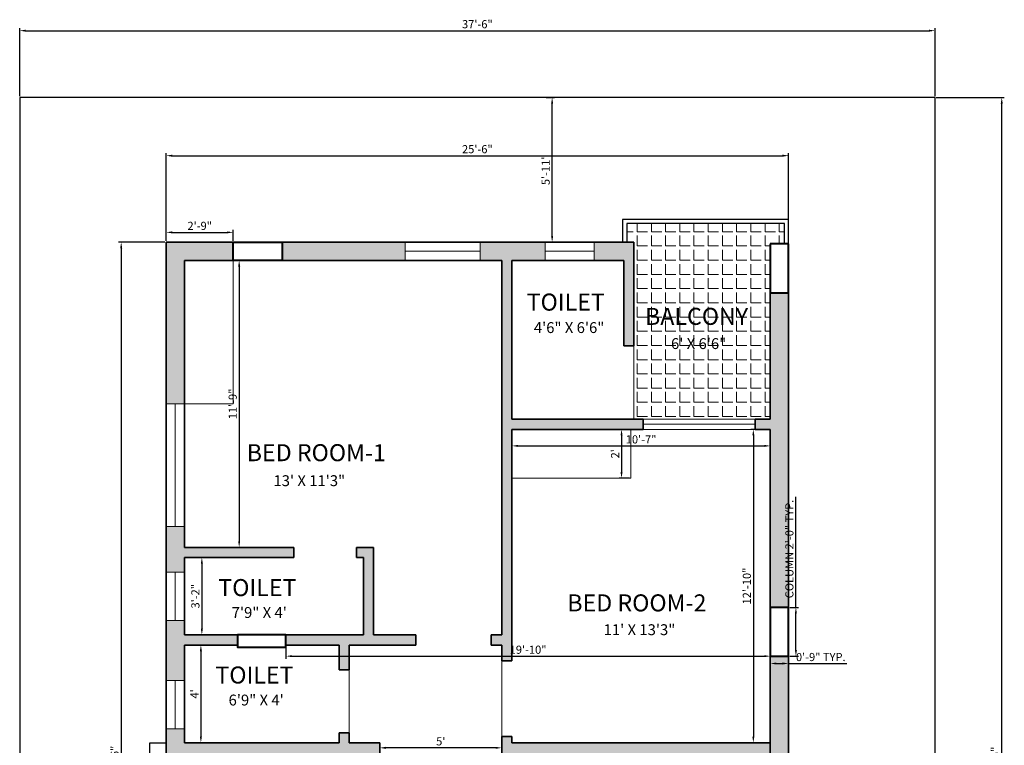
# Model space of a CAD drawing. Units: millimetres. Extents: x 2190 to 2674, y 1487 to 2179.
# Tile 2 of 2: x 2190 to 2674, y 1822 to 2179. Entities that reach past the tile are written whole.
import ezdxf

# ---------------------------------------------------------------- set-up
doc = ezdxf.new("R2010")
doc.units = ezdxf.units.MM
for name, color, linetype, lineweight in [('A-ANNO-DIMS', 2, 'Continuous', 18), ('A-AREA-IDEN', 7, 'Continuous', 18), ('A-WALL', 7, 'Continuous', 35), ('C-PROP', 7, 'Continuous', 25)]:
    doc.layers.add(name, color=color, linetype=linetype, lineweight=lineweight)
for name, color, linetype, lineweight, true_color in [('A-COLS', 240, 'Continuous', 40, 0xed1f24), ('A-DOOR', 177, 'Continuous', 18, 0x293189), ('A-FLOR-CASE', 177, 'Continuous', 18, 0x293189), ('A-FLOR-HRAL', 177, 'Continuous', 25, 0x293189), ('A-FLOR-PATT', 252, 'Continuous', 13, 0x939598), ('A-GLAZ', 177, 'Continuous', 18, 0x293189), ('A-WALL-PATT', 32, 'Continuous', 13, 0xcd6928)]:
    doc.layers.add(name, color=color, linetype=linetype, lineweight=lineweight, true_color=true_color)
doc.styles.get("Standard").update_dxf_attribs({"font": 'arial.ttf'})
doc.dimstyles.new('ISO-25', dxfattribs={"dimtxt": 4, "dimasz": 3, "dimexe": 1.25, "dimexo": 0.625, "dimtad": 1, "dimdec": 0, "dimlunit": 3, "dimtxsty": 'Standard', "dimcen": 2.5, "dimadec": 0, "dimazin": 0, "dimtfac": 1, "dimtdec": 0, "dimtmove": 0, "dimatfit": 3, "dimfxl": 1, "dimarcsym": 0})

# ---------------------------------------------------------------- blocks, each defined once
blk = doc.blocks.new('*D1')
at = {"layer": 'A-ANNO-DIMS', "color": 0, "lineweight": -2, "transparency": 16777216}
for p, q in [((2295.73, 2060.45), (2299.26, 2060.45)), ((2298.01, 2057.45), (2298.01, 1922.45)), ((2295.73, 1919.45), (2299.26, 1919.45))]:
    blk.add_line(p, q, dxfattribs=at)
at = {"layer": 'A-ANNO-DIMS', "color": 0, "transparency": 16777216}
for points in [[(2297.51, 2057.45), (2298.51, 2057.45), (2298.01, 2060.45)], [(2297.51, 1922.45), (2298.51, 1922.45), (2298.01, 1919.45)]]:
    blk.add_solid(points, dxfattribs=at)
at = {"layer": 'Defpoints', "color": 0, "transparency": 16777216}
for p in [(2295.11, 2060.45), (2295.11, 1919.45), (2298.01, 1919.45)]:
    blk.add_point(p, dxfattribs=at)
at = {"layer": 'A-ANNO-DIMS', "color": 0, "transparency": 16777216, "insert": (2295.35, 1989.95), "char_height": 4, "attachment_point": 5, "rotation": 90}
blk.add_mtext('11\'-9"', dxfattribs=at)
blk = doc.blocks.new('*D2')
at = {"layer": 'A-ANNO-DIMS', "color": 0, "lineweight": -2, "transparency": 16777216}
for p, q in [((2271.73, 1914.45), (2280.92, 1914.45)), ((2279.67, 1911.45), (2279.67, 1879.45)), ((2271.73, 1876.45), (2280.92, 1876.45))]:
    blk.add_line(p, q, dxfattribs=at)
at = {"layer": 'A-ANNO-DIMS', "color": 0, "transparency": 16777216}
for points in [[(2279.17, 1911.45), (2280.17, 1911.45), (2279.67, 1914.45)], [(2279.17, 1879.45), (2280.17, 1879.45), (2279.67, 1876.45)]]:
    blk.add_solid(points, dxfattribs=at)
at = {"layer": 'Defpoints', "color": 0, "transparency": 16777216}
for p in [(2271.11, 1914.45), (2271.11, 1876.45), (2279.67, 1876.45)]:
    blk.add_point(p, dxfattribs=at)
at = {"layer": 'A-ANNO-DIMS', "color": 0, "transparency": 16777216, "insert": (2277, 1895.45), "char_height": 4, "attachment_point": 5, "rotation": 90}
blk.add_mtext('3\'-2"', dxfattribs=at)
blk = doc.blocks.new('*D3')
at = {"layer": 'A-ANNO-DIMS', "color": 0, "lineweight": -2, "transparency": 16777216}
for p, q in [((2271.73, 1871.45), (2280.44, 1871.45)), ((2279.19, 1868.45), (2279.19, 1826.45)), ((2271.73, 1823.45), (2280.44, 1823.45))]:
    blk.add_line(p, q, dxfattribs=at)
at = {"layer": 'A-ANNO-DIMS', "color": 0, "transparency": 16777216}
for points in [[(2278.69, 1868.45), (2279.69, 1868.45), (2279.19, 1871.45)], [(2278.69, 1826.45), (2279.69, 1826.45), (2279.19, 1823.45)]]:
    blk.add_solid(points, dxfattribs=at)
at = {"layer": 'Defpoints', "color": 0, "transparency": 16777216}
for p in [(2271.11, 1871.45), (2271.11, 1823.45), (2279.19, 1823.45)]:
    blk.add_point(p, dxfattribs=at)
at = {"layer": 'A-ANNO-DIMS', "color": 0, "transparency": 16777216, "insert": (2276.57, 1847.45), "char_height": 4, "attachment_point": 5, "rotation": 90}
blk.add_mtext("4'", dxfattribs=at)
blk = doc.blocks.new('*D14')
at = {"layer": 'A-ANNO-DIMS', "color": 0, "lineweight": -2, "transparency": 16777216}
for p, q in [((2367.11, 1819.07), (2367.11, 1822.2)), ((2424.11, 1820.95), (2370.11, 1820.95)), ((2427.11, 1819.07), (2427.11, 1822.2))]:
    blk.add_line(p, q, dxfattribs=at)
at = {"layer": 'A-ANNO-DIMS', "color": 0, "transparency": 16777216}
for points in [[(2370.11, 1821.45), (2370.11, 1820.45), (2367.11, 1820.95)], [(2424.11, 1821.45), (2424.11, 1820.45), (2427.11, 1820.95)]]:
    blk.add_solid(points, dxfattribs=at)
at = {"layer": 'Defpoints', "color": 0, "transparency": 16777216}
for p in [(2367.11, 1820.95), (2367.11, 1818.45), (2427.11, 1818.45)]:
    blk.add_point(p, dxfattribs=at)
at = {"layer": 'A-ANNO-DIMS', "color": 0, "transparency": 16777216, "insert": (2397.11, 1823.61), "char_height": 4, "attachment_point": 5}
blk.add_mtext("5'", dxfattribs=at)
blk = doc.blocks.new('*D15')
at = {"layer": 'A-ANNO-DIMS', "color": 0, "lineweight": -2, "transparency": 16777216}
for p, q in [((2558.48, 1977.45), (2549.53, 1977.45)), ((2550.78, 1974.45), (2550.78, 1826.45)), ((2558.48, 1823.45), (2549.53, 1823.45))]:
    blk.add_line(p, q, dxfattribs=at)
at = {"layer": 'A-ANNO-DIMS', "color": 0, "transparency": 16777216}
for points in [[(2550.28, 1974.45), (2551.28, 1974.45), (2550.78, 1977.45)], [(2550.28, 1826.45), (2551.28, 1826.45), (2550.78, 1823.45)]]:
    blk.add_solid(points, dxfattribs=at)
at = {"layer": 'Defpoints', "color": 0, "transparency": 16777216}
for p in [(2559.11, 1977.45), (2550.78, 1823.45), (2559.11, 1823.45)]:
    blk.add_point(p, dxfattribs=at)
at = {"layer": 'A-ANNO-DIMS', "color": 0, "transparency": 16777216, "insert": (2548.11, 1900.45), "char_height": 4, "attachment_point": 5, "rotation": 90}
blk.add_mtext('12\'-10"', dxfattribs=at)
blk = doc.blocks.new('*D16')
at = {"layer": 'A-ANNO-DIMS', "color": 0, "lineweight": -2, "transparency": 16777216}
for p, q in [((2432.11, 1976.82), (2432.11, 1968.07)), ((2559.11, 1976.82), (2559.11, 1968.07)), ((2435.11, 1969.32), (2556.11, 1969.32))]:
    blk.add_line(p, q, dxfattribs=at)
at = {"layer": 'A-ANNO-DIMS', "color": 0, "transparency": 16777216}
for points in [[(2435.11, 1969.82), (2435.11, 1968.82), (2432.11, 1969.32)], [(2556.11, 1969.82), (2556.11, 1968.82), (2559.11, 1969.32)]]:
    blk.add_solid(points, dxfattribs=at)
at = {"layer": 'Defpoints', "color": 0, "transparency": 16777216}
for p in [(2432.11, 1977.45), (2559.11, 1977.45), (2559.11, 1969.32)]:
    blk.add_point(p, dxfattribs=at)
at = {"layer": 'A-ANNO-DIMS', "color": 0, "transparency": 16777216, "insert": (2495.61, 1971.99), "char_height": 4, "width": 10.0232, "attachment_point": 5}
blk.add_mtext('10\'-7"', dxfattribs=at)
blk = doc.blocks.new('*D17')
at = {"layer": 'A-ANNO-DIMS', "color": 0, "lineweight": -2, "transparency": 16777216}
for p, q in [((2489.89, 1977.45), (2484.74, 1977.45)), ((2485.99, 1974.45), (2485.99, 1956.45)), ((2489.89, 1953.45), (2484.74, 1953.45))]:
    blk.add_line(p, q, dxfattribs=at)
at = {"layer": 'A-ANNO-DIMS', "color": 0, "transparency": 16777216}
for points in [[(2485.49, 1974.45), (2486.49, 1974.45), (2485.99, 1977.45)], [(2485.49, 1956.45), (2486.49, 1956.45), (2485.99, 1953.45)]]:
    blk.add_solid(points, dxfattribs=at)
at = {"layer": 'Defpoints', "color": 0, "transparency": 16777216}
for p in [(2490.51, 1977.45), (2485.99, 1953.45), (2490.51, 1953.45)]:
    blk.add_point(p, dxfattribs=at)
at = {"layer": 'A-ANNO-DIMS', "color": 0, "transparency": 16777216, "insert": (2483.36, 1965.45), "char_height": 4, "attachment_point": 5, "rotation": 90}
blk.add_mtext("2'", dxfattribs=at)
blk = doc.blocks.new('*D18')
at = {"layer": 'A-ANNO-DIMS', "color": 0, "lineweight": -2, "transparency": 16777216}
for p, q in [((2262.11, 2070.07), (2262.11, 2075.5)), ((2265.11, 2074.25), (2292.11, 2074.25)), ((2295.11, 2070.07), (2295.11, 2075.5))]:
    blk.add_line(p, q, dxfattribs=at)
at = {"layer": 'A-ANNO-DIMS', "color": 0, "transparency": 16777216}
for points in [[(2265.11, 2074.75), (2265.11, 2073.75), (2262.11, 2074.25)], [(2292.11, 2074.75), (2292.11, 2073.75), (2295.11, 2074.25)]]:
    blk.add_solid(points, dxfattribs=at)
at = {"layer": 'Defpoints', "color": 0, "transparency": 16777216}
for p in [(2295.11, 2074.25), (2262.11, 2069.45), (2295.11, 2069.45)]:
    blk.add_point(p, dxfattribs=at)
at = {"layer": 'A-ANNO-DIMS', "color": 0, "transparency": 16777216, "insert": (2278.61, 2076.92), "char_height": 4, "attachment_point": 5}
blk.add_mtext('2\'-9"', dxfattribs=at)
blk = doc.blocks.new('*D19')
at = {"layer": 'A-ANNO-DIMS', "color": 0, "lineweight": -2, "transparency": 16777216}
for p, q in [((2320.99, 1870.82), (2320.99, 1864.74)), ((2559.11, 1870.82), (2559.11, 1864.74)), ((2323.99, 1865.99), (2556.11, 1865.99))]:
    blk.add_line(p, q, dxfattribs=at)
at = {"layer": 'A-ANNO-DIMS', "color": 0, "transparency": 16777216}
for points in [[(2323.99, 1866.49), (2323.99, 1865.49), (2320.99, 1865.99)], [(2556.11, 1866.49), (2556.11, 1865.49), (2559.11, 1865.99)]]:
    blk.add_solid(points, dxfattribs=at)
at = {"layer": 'Defpoints', "color": 0, "transparency": 16777216}
for p in [(2320.99, 1871.45), (2559.11, 1871.45), (2559.11, 1865.99)]:
    blk.add_point(p, dxfattribs=at)
at = {"layer": 'A-ANNO-DIMS', "color": 0, "transparency": 16777216, "insert": (2440.05, 1868.65), "char_height": 4, "attachment_point": 5}
blk.add_mtext('19\'-10"', dxfattribs=at)
blk = doc.blocks.new('*D20')
at = {"layer": 'A-ANNO-DIMS', "color": 0, "lineweight": -2, "transparency": 16777216}
for p, q in [((2262.11, 2070.07), (2262.11, 2113.18)), ((2265.11, 2111.93), (2565.11, 2111.93)), ((2568.11, 2069.18), (2568.11, 2113.18))]:
    blk.add_line(p, q, dxfattribs=at)
at = {"layer": 'A-ANNO-DIMS', "color": 0, "transparency": 16777216}
for points in [[(2265.11, 2112.43), (2265.11, 2111.43), (2262.11, 2111.93)], [(2565.11, 2112.43), (2565.11, 2111.43), (2568.11, 2111.93)]]:
    blk.add_solid(points, dxfattribs=at)
at = {"layer": 'Defpoints', "color": 0, "transparency": 16777216}
for p in [(2568.11, 2111.93), (2262.11, 2069.45), (2568.11, 2068.55)]:
    blk.add_point(p, dxfattribs=at)
at = {"layer": 'A-ANNO-DIMS', "color": 0, "transparency": 16777216, "insert": (2415.11, 2114.6), "char_height": 4, "attachment_point": 5}
blk.add_mtext('25\'-6"', dxfattribs=at)
blk = doc.blocks.new('*D21')
at = {"layer": 'A-ANNO-DIMS', "color": 0, "lineweight": -2, "transparency": 16777216}
for p, q in [((2261.48, 2069.45), (2238.76, 2069.45)), ((2240.01, 2066.45), (2240.01, 1562.45)), ((2261.48, 1559.45), (2238.76, 1559.45))]:
    blk.add_line(p, q, dxfattribs=at)
at = {"layer": 'A-ANNO-DIMS', "color": 0, "transparency": 16777216}
for points in [[(2239.51, 2066.45), (2240.51, 2066.45), (2240.01, 2069.45)], [(2239.51, 1562.45), (2240.51, 1562.45), (2240.01, 1559.45)]]:
    blk.add_solid(points, dxfattribs=at)
at = {"layer": 'Defpoints', "color": 0, "transparency": 16777216}
for p in [(2262.11, 2069.45), (2240.01, 1559.45), (2262.11, 1559.45)]:
    blk.add_point(p, dxfattribs=at)
at = {"layer": 'A-ANNO-DIMS', "color": 0, "transparency": 16777216, "insert": (2237.34, 1814.45), "char_height": 4, "attachment_point": 5, "rotation": 90}
blk.add_mtext('42\'-6"', dxfattribs=at)
blk = doc.blocks.new('*D25')
at = {"layer": 'A-ANNO-DIMS', "color": 0, "lineweight": -2, "transparency": 16777216}
for p, q in [((2449.01, 2140.55), (2453.11, 2140.55)), ((2451.86, 2072.45), (2451.86, 2137.55)), ((2449.01, 2069.45), (2453.11, 2069.45))]:
    blk.add_line(p, q, dxfattribs=at)
at = {"layer": 'A-ANNO-DIMS', "color": 0, "transparency": 16777216}
for points in [[(2451.36, 2137.55), (2452.36, 2137.55), (2451.86, 2140.55)], [(2451.36, 2072.45), (2452.36, 2072.45), (2451.86, 2069.45)]]:
    blk.add_solid(points, dxfattribs=at)
at = {"layer": 'Defpoints', "color": 0, "transparency": 16777216}
for p in [(2448.39, 2140.55), (2451.86, 2140.55), (2448.39, 2069.45)]:
    blk.add_point(p, dxfattribs=at)
at = {"layer": 'A-ANNO-DIMS', "color": 0, "transparency": 16777216, "insert": (2449.2, 2105), "char_height": 4, "attachment_point": 5, "rotation": 90}
blk.add_mtext('5\'-11"', dxfattribs=at)
blk = doc.blocks.new('COLUMN-RECT-LONG-Y')
for p, q in [((9, 24), (0, 24)), ((0, 24), (0, 0)), ((9, 0), (9, 24)), ((0, 0), (9, 0))]:
    blk.add_line(p, q)
blk = doc.blocks.new('*D28')
at = {"layer": 'A-ANNO-DIMS', "color": 0, "lineweight": -2, "transparency": 16777216}
for p, q in [((2571.71, 1889.99), (2571.71, 1944.34)), ((2568.73, 1889.99), (2572.96, 1889.99)), ((2571.71, 1868.99), (2571.71, 1886.99)), ((2568.73, 1865.99), (2572.96, 1865.99))]:
    blk.add_line(p, q, dxfattribs=at)
at = {"layer": 'A-ANNO-DIMS', "color": 0, "transparency": 16777216}
for points in [[(2571.21, 1886.99), (2572.21, 1886.99), (2571.71, 1889.99)], [(2571.21, 1868.99), (2572.21, 1868.99), (2571.71, 1865.99)]]:
    blk.add_solid(points, dxfattribs=at)
at = {"layer": 'Defpoints', "color": 0, "transparency": 16777216}
for p in [(2568.11, 1889.99), (2571.71, 1889.99), (2568.11, 1865.99)]:
    blk.add_point(p, dxfattribs=at)
at = {"layer": 'A-ANNO-DIMS', "color": 0, "transparency": 16777216, "insert": (2569.02, 1918.66), "char_height": 4, "attachment_point": 5, "rotation": 90}
blk.add_mtext('COLUMN 2\'-0" TYP.', dxfattribs=at)
blk = doc.blocks.new('*D29')
at = {"layer": 'A-ANNO-DIMS', "color": 0, "lineweight": -2, "transparency": 16777216}
for p, q in [((2559.11, 1865.36), (2559.11, 1861.14)), ((2568.11, 1865.36), (2568.11, 1861.14)), ((2562.11, 1862.39), (2565.11, 1862.39)), ((2568.11, 1862.39), (2596.74, 1862.39))]:
    blk.add_line(p, q, dxfattribs=at)
at = {"layer": 'A-ANNO-DIMS', "color": 0, "transparency": 16777216}
for points in [[(2562.11, 1862.89), (2562.11, 1861.89), (2559.11, 1862.39)], [(2565.11, 1862.89), (2565.11, 1861.89), (2568.11, 1862.39)]]:
    blk.add_solid(points, dxfattribs=at)
at = {"layer": 'Defpoints', "color": 0, "transparency": 16777216}
for p in [(2559.11, 1865.99), (2568.11, 1865.99), (2568.11, 1862.39)]:
    blk.add_point(p, dxfattribs=at)
at = {"layer": 'A-ANNO-DIMS', "color": 0, "transparency": 16777216, "insert": (2583.93, 1865.05), "char_height": 4, "attachment_point": 5}
blk.add_mtext('0\'-9" TYP.', dxfattribs=at)
blk = doc.blocks.new('*D32')
at = {"layer": 'A-ANNO-DIMS', "color": 0, "lineweight": -2, "transparency": 16777216}
for p, q in [((2190.11, 2141.18), (2190.11, 2174.6)), ((2640.11, 2141.18), (2640.11, 2174.6)), ((2193.11, 2173.35), (2637.11, 2173.35))]:
    blk.add_line(p, q, dxfattribs=at)
at = {"layer": 'A-ANNO-DIMS', "color": 0, "transparency": 16777216}
for points in [[(2193.11, 2173.85), (2193.11, 2172.85), (2190.11, 2173.35)], [(2637.11, 2173.85), (2637.11, 2172.85), (2640.11, 2173.35)]]:
    blk.add_solid(points, dxfattribs=at)
at = {"layer": 'Defpoints', "color": 0, "transparency": 16777216}
for p in [(2640.11, 2173.35), (2190.11, 2140.55), (2640.11, 2140.55)]:
    blk.add_point(p, dxfattribs=at)
at = {"layer": 'A-ANNO-DIMS', "color": 0, "transparency": 16777216, "insert": (2415.11, 2176.02), "char_height": 4, "attachment_point": 5}
blk.add_mtext('37\'-6"', dxfattribs=at)
blk = doc.blocks.new('*D33')
at = {"layer": 'A-ANNO-DIMS', "color": 0, "lineweight": -2, "transparency": 16777216}
for p, q in [((2640.73, 2140.55), (2674.16, 2140.55)), ((2672.91, 1490.45), (2672.91, 2137.55)), ((2640.73, 1487.45), (2674.16, 1487.45))]:
    blk.add_line(p, q, dxfattribs=at)
at = {"layer": 'A-ANNO-DIMS', "color": 0, "transparency": 16777216}
for points in [[(2672.41, 2137.55), (2673.41, 2137.55), (2672.91, 2140.55)], [(2672.41, 1490.45), (2673.41, 1490.45), (2672.91, 1487.45)]]:
    blk.add_solid(points, dxfattribs=at)
at = {"layer": 'Defpoints', "color": 0, "transparency": 16777216}
for p in [(2640.11, 2140.55), (2672.91, 2140.55), (2640.11, 1487.45)]:
    blk.add_point(p, dxfattribs=at)
at = {"layer": 'A-ANNO-DIMS', "color": 0, "transparency": 16777216, "insert": (2670.25, 1814), "char_height": 4, "attachment_point": 5, "rotation": 90}
blk.add_mtext('54\'-5"', dxfattribs=at)

msp = doc.modelspace()

# ---------------------------------------------------------------- hatches: boundary and pattern name
at = {"layer": 'A-FLOR-PATT'}
h = msp.add_hatch(dxfattribs=at)
h.set_pattern_fill('ANGLE', color=256)
h.set_pattern_definition([(0, (0, 0), (0, 6.985), [5.08, -1.905]), (90, (0, 0), (-6.985, 4e-16), [5.08, -1.905])])
h.paths.add_polyline_path([(2559.11, 2060.45), (2559.11, 2068.55), (2566.11, 2068.55), (2566.11, 2078.55), (2488.53, 2078.55), (2488.53, 2069.45), (2492.11, 2069.45), (2492.11, 2060.45), (2492.11, 2018.45), (2492.11, 1982.45), (2496.64, 1982.45), (2551.7, 1982.45), (2559.11, 1982.45)])
h.paths.add_polyline_path([(2508.94, 2015.46), (2538.79, 2015.46), (2538.79, 2023.66), (2508.94, 2023.66)], flags=24)
h.paths.add_polyline_path([(2495.36, 2026.48), (2555.55, 2026.48), (2555.55, 2039.46), (2495.36, 2039.46)], flags=24)
at = {"layer": 'A-WALL-PATT'}
h = msp.add_hatch(color=256, dxfattribs=at)
h.dxf.hatch_style = 1
h.paths.add_polyline_path([(2295.11, 2069.45), (2262.11, 2069.45), (2262.11, 2060.45), (2262.11, 1989.95), (2271.11, 1989.95), (2271.11, 2060.45), (2295.11, 2060.45)])
h.paths.add_polyline_path([(2379.55, 2069.45), (2319.11, 2069.45), (2319.11, 2060.45), (2379.55, 2060.45)])
h.paths.add_polyline_path([(2448.39, 2069.45), (2433.11, 2069.45), (2416.52, 2069.45), (2416.52, 2060.45), (2427.11, 2060.45), (2427.11, 1919.45), (2427.11, 1876.45), (2421.86, 1876.45), (2421.86, 1871.45), (2427.11, 1871.45), (2427.11, 1863.71), (2432.11, 1863.71), (2432.11, 1919.45), (2432.11, 1977.45), (2496.64, 1977.45), (2496.64, 1982.45), (2492.11, 1982.45), (2487.11, 1982.45), (2432.11, 1982.45), (2432.11, 2060.45), (2433.11, 2060.45), (2448.39, 2060.45)])
h.paths.add_polyline_path([(2492.11, 2069.45), (2487.11, 2069.45), (2472.59, 2069.45), (2472.59, 2060.45), (2487.11, 2060.45), (2487.11, 2018.45), (2492.11, 2018.45), (2492.11, 2060.45)], flags=17)
h.paths.add_polyline_path([(2568.11, 1823.45), (2568.11, 1865.99), (2559.11, 1865.99), (2559.11, 1823.45), (2559.11, 1735.69), (2568.11, 1735.69)])
h.paths.add_polyline_path([(2559.11, 1823.45), (2432.11, 1823.45), (2432.11, 1826.45), (2427.11, 1826.45), (2427.11, 1823.45), (2427.11, 1818.45), (2559.11, 1818.45)])
h.paths.add_polyline_path([(2568.11, 1982.45), (2568.11, 2044.55), (2559.11, 2044.55), (2559.11, 1982.45), (2551.7, 1982.45), (2551.7, 1977.45), (2559.11, 1977.45), (2559.11, 1889.99), (2568.11, 1889.99)])
h.paths.add_polyline_path([(2352.11, 1871.45), (2384.83, 1871.45), (2384.83, 1876.45), (2364.11, 1876.45), (2364.11, 1919.45), (2355.61, 1919.45), (2355.61, 1914.45), (2359.11, 1914.45), (2359.11, 1876.45), (2320.99, 1876.45), (2320.99, 1871.45), (2347.11, 1871.45), (2347.11, 1859.22), (2352.11, 1859.22)])
h.paths.add_polyline_path([(2297.23, 1876.45), (2271.11, 1876.45), (2271.11, 1883.52), (2262.11, 1883.52), (2262.11, 1871.45), (2262.11, 1854.01), (2271.11, 1854.01), (2271.11, 1871.45), (2297.23, 1871.45)])
h.paths.add_polyline_path([(2367.11, 1823.45), (2352.11, 1823.45), (2352.11, 1828.35), (2347.11, 1828.35), (2347.11, 1823.45), (2271.11, 1823.45), (2271.11, 1830.23), (2262.11, 1830.23), (2262.11, 1823.45), (2262.11, 1818.45), (2271.11, 1818.45), (2299.11, 1818.45), (2299.11, 1793.58), (2304.11, 1793.58), (2304.11, 1818.45), (2367.11, 1818.45)])
h.paths.add_polyline_path([(2271.11, 1929.68), (2262.11, 1929.68), (2262.11, 1919.45), (2262.11, 1907.21), (2271.11, 1907.21), (2271.11, 1914.45), (2324.92, 1914.45), (2324.92, 1919.45), (2271.11, 1919.45)])
h.paths.add_polyline_path([(2299.11, 1690.45), (2271.11, 1690.45), (2262.11, 1690.45), (2262.11, 1685.45), (2262.11, 1653.98), (2271.11, 1653.98), (2271.11, 1685.45), (2296.11, 1685.45), (2299.11, 1685.45), (2299.11, 1686.45)])
h.paths.add_polyline_path([(2304.11, 1709.13), (2299.11, 1709.13), (2299.11, 1690.45), (2304.11, 1690.45)])
h.paths.add_polyline_path([(2299.11, 1568.45), (2271.11, 1568.45), (2271.11, 1592.45), (2271.11, 1593.45), (2271.11, 1618.52), (2262.11, 1618.52), (2262.11, 1568.45), (2262.11, 1559.45), (2271.11, 1559.45), (2299.11, 1559.45), (2299.11, 1564.45)])
h.paths.add_polyline_path([(2366.54, 1568.45), (2323.11, 1568.45), (2323.11, 1559.45), (2366.54, 1559.45)])
h.paths.add_polyline_path([(2493.88, 1568.45), (2421.11, 1568.45), (2421.11, 1593.45), (2421.11, 1685.45), (2502.11, 1685.45), (2502.11, 1690.45), (2421.11, 1690.45), (2416.11, 1690.45), (2416.11, 1685.45), (2416.11, 1648.45), (2373.11, 1648.45), (2373.11, 1690.45), (2368.11, 1690.45), (2368.11, 1648.45), (2368.11, 1643.45), (2373.11, 1643.45), (2416.11, 1643.45), (2416.11, 1568.45), (2403.74, 1568.45), (2403.74, 1559.45), (2421.11, 1559.45), (2493.88, 1559.45)])
h.paths.add_polyline_path([(2559.11, 1568.45), (2543.07, 1568.45), (2543.07, 1559.45), (2559.11, 1559.45)])
h.paths.add_polyline_path([(2568.11, 1666.45), (2559.11, 1666.45), (2559.11, 1583.45), (2568.11, 1583.45)])
h.paths.add_polyline_path([(2559.11, 1690.45), (2538.11, 1690.45), (2538.11, 1685.45), (2559.11, 1685.45)])
h.paths.add_polyline_path([(2568.11, 1699.69), (2559.11, 1699.69), (2559.11, 1690.45), (2568.11, 1690.45)])

# ---------------------------------------------------------------- linework, layer by layer
at = {"layer": 'A-COLS'}
msp.add_lwpolyline([(2295.11, 2069.45), (2319.11, 2069.45), (2319.11, 2060.45), (2295.11, 2060.45)], close=True, dxfattribs=at)
for points in [[(2309.11, 1876.45), (2297.23, 1876.45), (2297.23, 1870.49), (2309.11, 1870.49)], [(2309.11, 1870.49), (2320.99, 1870.49), (2320.99, 1876.45), (2309.11, 1876.45)]]:
    msp.add_lwpolyline(points, dxfattribs=at)
at = {"layer": 'A-DOOR'}
for p, q in [((2492.11, 2018.45), (2492.11, 1982.45)), ((2427.11, 1863.71), (2427.11, 1826.45)), ((2352.11, 1859.22), (2352.11, 1828.35))]:
    msp.add_line(p, q, dxfattribs=at)
at = {"layer": 'A-FLOR-CASE'}
for p, q in [((2295.11, 2060.45), (2295.11, 1989.95)), ((2295.11, 1989.95), (2271.11, 1989.95)), ((2490.51, 1953.45), (2490.51, 1977.45)), ((2432.11, 1953.45), (2490.51, 1953.45))]:
    msp.add_line(p, q, dxfattribs=at)
at = {"layer": 'A-FLOR-HRAL'}
for p, q in [((2568.11, 2080.55), (2486.53, 2080.55)), ((2486.53, 2080.55), (2486.53, 2069.45)), ((2566.11, 2078.55), (2488.53, 2078.55)), ((2488.53, 2078.55), (2488.53, 2069.45)), ((2566.11, 2068.55), (2566.11, 2078.55)), ((2568.11, 2068.55), (2568.11, 2080.55)), ((2254.11, 1686.04), (2254.11, 1823.45)), ((2254.11, 1823.45), (2262.11, 1823.45))]:
    msp.add_line(p, q, dxfattribs=at)
at = {"layer": 'A-GLAZ'}
for p, q in [((2379.55, 2064.95), (2416.52, 2064.95)), ((2448.39, 2064.95), (2472.59, 2064.95)), ((2266.61, 1989.95), (2266.61, 1929.68)), ((2496.64, 1979.95), (2551.7, 1979.95)), ((2266.61, 1907.21), (2266.61, 1883.52)), ((2266.61, 1854.01), (2266.61, 1830.23))]:
    msp.add_line(p, q, dxfattribs=at)
for points in [[(2416.52, 2060.45), (2379.55, 2060.45), (2379.55, 2069.45), (2416.52, 2069.45)], [(2271.11, 1929.68), (2262.11, 1929.68), (2262.11, 1989.95), (2271.11, 1989.95)], [(2496.64, 1982.45), (2551.7, 1982.45), (2551.7, 1977.45), (2496.64, 1977.45)], [(2271.11, 1830.23), (2262.11, 1830.23), (2262.11, 1854.01), (2271.11, 1854.01)]]:
    msp.add_lwpolyline(points, close=True, dxfattribs=at)
for points in [[(2460.11, 2060.45), (2448.39, 2060.45), (2448.39, 2069.45), (2460.11, 2069.45)], [(2460.11, 2060.45), (2472.59, 2060.45), (2472.59, 2069.45), (2460.11, 2069.45)], [(2262.11, 1895.45), (2262.11, 1907.21), (2271.11, 1907.21), (2271.11, 1895.45)], [(2262.11, 1895.45), (2262.11, 1883.52), (2271.11, 1883.52), (2271.11, 1895.45)]]:
    msp.add_lwpolyline(points, dxfattribs=at)
at = {"layer": 'A-WALL'}
for p, q in [((2262.11, 2060.45), (2262.11, 2069.45)), ((2271.11, 2069.45), (2262.11, 2069.45)), ((2262.11, 2069.45), (2295.11, 2069.45)), ((2271.11, 2069.45), (2433.11, 2069.45)), ((2295.11, 2069.45), (2295.11, 2060.45)), ((2319.11, 2060.45), (2319.11, 2069.45)), ((2487.11, 2069.45), (2433.11, 2069.45)), ((2487.11, 2069.45), (2492.11, 2069.45)), ((2492.11, 2060.45), (2492.11, 2069.45)), ((2559.11, 2068.55), (2559.11, 2060.45)), ((2568.11, 2060.45), (2568.11, 2068.55)), ((2262.11, 2060.45), (2262.11, 1919.45)), ((2271.11, 2060.45), (2427.11, 2060.45)), ((2271.11, 2060.45), (2271.11, 1919.45)), ((2295.11, 2060.45), (2319.11, 2060.45)), ((2427.11, 2060.45), (2427.11, 1919.45)), ((2432.11, 2060.45), (2432.11, 1982.45)), ((2432.11, 2060.45), (2433.11, 2060.45)), ((2487.11, 2060.45), (2433.11, 2060.45)), ((2487.11, 2060.45), (2487.11, 2018.45)), ((2492.11, 2060.45), (2492.11, 2018.45)), ((2559.11, 1982.45), (2559.11, 2060.45)), ((2568.11, 1982.45), (2568.11, 2060.45)), ((2487.11, 1982.45), (2432.11, 1982.45)), ((2496.64, 1982.45), (2492.11, 1982.45)), ((2559.11, 1982.45), (2551.7, 1982.45)), ((2568.11, 1823.45), (2568.11, 1982.45)), ((2432.11, 1977.45), (2432.11, 1919.45)), ((2496.64, 1977.45), (2432.11, 1977.45)), ((2432.11, 1977.45), (2432.11, 1953.45)), ((2559.11, 1977.45), (2551.7, 1977.45)), ((2559.11, 1823.45), (2559.11, 1977.45)), ((2262.11, 1871.45), (2262.11, 1919.45)), ((2271.11, 1919.45), (2324.92, 1919.45)), ((2364.11, 1919.45), (2355.61, 1919.45)), ((2364.11, 1876.45), (2364.11, 1919.45)), ((2427.11, 1876.45), (2427.11, 1919.45)), ((2432.11, 1863.71), (2432.11, 1919.45)), ((2271.11, 1876.45), (2271.11, 1914.45)), ((2271.11, 1914.45), (2324.92, 1914.45)), ((2359.11, 1914.45), (2355.61, 1914.45)), ((2359.11, 1876.45), (2359.11, 1914.45)), ((2271.11, 1876.45), (2359.11, 1876.45)), ((2364.11, 1876.45), (2384.83, 1876.45)), ((2421.86, 1876.45), (2427.11, 1876.45)), ((2262.11, 1871.45), (2262.11, 1823.45)), ((2271.11, 1871.45), (2271.11, 1823.45)), ((2271.11, 1871.45), (2297.23, 1871.45)), ((2297.23, 1871.45), (2271.11, 1871.45)), ((2347.11, 1871.45), (2320.99, 1871.45)), ((2320.99, 1871.45), (2347.11, 1871.45)), ((2347.11, 1859.22), (2347.11, 1871.45)), ((2352.11, 1871.45), (2384.83, 1871.45)), ((2352.11, 1859.22), (2352.11, 1871.45)), ((2421.86, 1871.45), (2427.11, 1871.45)), ((2427.11, 1863.71), (2427.11, 1871.45)), ((2347.11, 1823.45), (2347.11, 1828.35)), ((2352.11, 1823.45), (2352.11, 1828.35)), ((2427.11, 1823.45), (2427.11, 1826.45)), ((2432.11, 1823.45), (2432.11, 1826.45)), ((2262.11, 1823.45), (2262.11, 1818.45)), ((2271.11, 1823.45), (2347.11, 1823.45)), ((2271.11, 1823.45), (2304.11, 1823.45)), ((2352.11, 1823.45), (2367.11, 1823.45)), ((2559.11, 1823.45), (2432.11, 1823.45)), ((2559.11, 1735.69), (2559.11, 1823.45)), ((2568.11, 1735.69), (2568.11, 1823.45))]:
    msp.add_line(p, q, dxfattribs=at)
for points in [[(2487.11, 2018.45), (2492.11, 2018.45)], [(2492.11, 1982.45), (2487.11, 1982.45)], [(2496.64, 1977.45), (2496.64, 1982.45)], [(2551.7, 1982.45), (2551.7, 1977.45)], [(2324.92, 1914.45), (2324.92, 1919.45)], [(2355.61, 1919.45), (2355.61, 1914.45)], [(2384.83, 1871.45), (2384.83, 1876.45)], [(2421.86, 1876.45), (2421.86, 1871.45)], [(2427.11, 1863.71), (2432.11, 1863.71)], [(2347.11, 1859.22), (2352.11, 1859.22)], [(2352.11, 1828.35), (2347.11, 1828.35)], [(2432.11, 1826.45), (2427.11, 1826.45)], [(2367.11, 1823.45), (2367.11, 1818.45)], [(2427.11, 1818.45), (2427.11, 1823.45)]]:
    msp.add_lwpolyline(points, dxfattribs=at)
at = {"layer": 'C-PROP'}
for p, q in [((2262.11, 2140.55), (2190.11, 2140.55)), ((2190.11, 2140.55), (2190.11, 1559.45)), ((2568.11, 2140.55), (2262.11, 2140.55)), ((2640.11, 2140.55), (2568.11, 2140.55)), ((2640.11, 1487.45), (2640.11, 2140.55))]:
    msp.add_line(p, q, dxfattribs=at)

# ---------------------------------------------------------------- block references
at = {"layer": 'A-COLS'}
for p in [(2559.11, 2044.55), (2559.11, 1865.99)]:
    msp.add_blockref('COLUMN-RECT-LONG-Y', p, dxfattribs=at)

# ---------------------------------------------------------------- texts
at = {"layer": 'A-AREA-IDEN'}
for s, height, p in [('TOILET', 8.367, (2439.35, 2035.79)), ('BALCONY', 8.367, (2497.53, 2028.78)), ('4\'6" X 6\'6"', 5.3513, (2442.88, 2024.78)), ('6\' X 6\'6"', 5.351, (2510.31, 2016.92)), ('BED ROOM-1', 8.367, (2301.74, 1961.8)), ('13\' X 11\'3"', 5.3513, (2314.87, 1949.55)), ('TOILET', 8.367, (2287.74, 1895.5)), ('BED ROOM-2', 8.367, (2459.33, 1887.99)), ('7\'9" X 4\'', 5.351, (2294.34, 1884.77)), ('11\' X 13\'3"', 5.3513, (2477.18, 1876.32)), ('TOILET', 8.367, (2286.32, 1852.55)), ('6\'9" X 4\'', 5.351, (2292.8, 1841.76))]:
    msp.add_text(s, height=height, dxfattribs=at).set_placement(p)

# ---------------------------------------------------------------- dimensions: what is measured, and where the dimension line sits
at = {"layer": 'A-ANNO-DIMS'}
for base, p1, p2, override, picture, middle in [((2640.11, 2173.35), (2190.11, 2140.55), (2640.11, 2140.55), {"dimdec": 1, "dimlfac": 1, "dimrnd": 0, "dimzin": 1, "dimdsep": 46, "dimlunit": 4, "dimfrac": 2}, '*D32', (2415.11, 2176.02)), ((2568.11, 2111.93), (2262.11, 2069.45), (2568.11, 2068.55), {"dimclrd": 0, "dimclre": 0, "dimclrt": 0}, '*D20', (2415.11, 2114.6)), ((2295.11, 2074.25), (2262.11, 2069.45), (2295.11, 2069.45), {"dimclrd": 0, "dimclre": 0, "dimclrt": 0}, '*D18', (2278.61, 2076.92)), ((2559.11, 1969.32), (2432.11, 1977.45), (2559.11, 1977.45), {"dimclrd": 0, "dimclre": 0, "dimclrt": 0}, '*D16', (2495.61, 1971.99)), ((2559.11, 1865.99), (2320.99, 1871.45), (2559.11, 1871.45), {"dimclrd": 0, "dimclre": 0, "dimclrt": 0}, '*D19', (2440.05, 1868.65)), ((2367.11, 1820.95), (2427.11, 1818.45), (2367.11, 1818.45), {"dimclrd": 0, "dimclre": 0, "dimclrt": 0}, '*D14', (2397.11, 1823.61))]:
    dim = msp.add_linear_dim(base=base, p1=p1, p2=p2, dimstyle='ISO-25', override=override, dxfattribs=at)
    dim.commit()
    dim.dimension.update_dxf_attribs({"geometry": picture, "text_midpoint": middle})
for base, p1, p2, override, picture, middle in [((2451.86, 2140.55), (2448.39, 2069.45), (2448.39, 2140.55), {"dimclrd": 0, "dimclre": 0, "dimclrt": 0}, '*D25', (2449.2, 2105)), ((2672.91, 2140.55), (2640.11, 1487.45), (2640.11, 2140.55), {"dimdec": 1, "dimlfac": 1, "dimrnd": 0, "dimzin": 1, "dimdsep": 46, "dimlunit": 4, "dimfrac": 2}, '*D33', (2670.25, 1814)), ((2240.01, 1559.45), (2262.11, 2069.45), (2262.11, 1559.45), {"dimclrd": 0, "dimclre": 0, "dimclrt": 0}, '*D21', (2237.34, 1814.45)), ((2298.01, 1919.45), (2295.11, 2060.45), (2295.11, 1919.45), {"dimclrd": 0, "dimclre": 0, "dimclrt": 0}, '*D1', (2295.35, 1989.95)), ((2485.99, 1953.45), (2490.51, 1977.45), (2490.51, 1953.45), {"dimclrd": 0, "dimclre": 0, "dimclrt": 0}, '*D17', (2483.36, 1965.45)), ((2550.78, 1823.45), (2559.11, 1977.45), (2559.11, 1823.45), {"dimclrd": 0, "dimclre": 0, "dimclrt": 0}, '*D15', (2548.11, 1900.45)), ((2279.67, 1876.45), (2271.11, 1914.45), (2271.11, 1876.45), {"dimclrd": 0, "dimclre": 0, "dimclrt": 0}, '*D2', (2277, 1895.45)), ((2279.19, 1823.45), (2271.11, 1871.45), (2271.11, 1823.45), {"dimclrd": 0, "dimclre": 0, "dimclrt": 0}, '*D3', (2276.57, 1847.45))]:
    dim = msp.add_linear_dim(base=base, p1=p1, p2=p2, angle=90, dimstyle='ISO-25', override=override, dxfattribs=at)
    dim.commit()
    dim.dimension.update_dxf_attribs({"geometry": picture, "text_midpoint": middle})
dim = msp.add_linear_dim(base=(2571.71, 1889.99), p1=(2568.11, 1865.99), p2=(2568.11, 1889.99), angle=90, text='COLUMN <> TYP.', dimstyle='ISO-25', override={"dimdec": 1, "dimlfac": 1, "dimrnd": 0, "dimzin": 1, "dimdsep": 46, "dimlunit": 4, "dimfrac": 2}, dxfattribs=at)
dim.commit()
dim.dimension.update_dxf_attribs({"geometry": '*D28', "text_midpoint": (2569.02, 1918.66)})
dim = msp.add_linear_dim(base=(2568.11, 1862.39), p1=(2559.11, 1865.99), p2=(2568.11, 1865.99), text='<> TYP.', dimstyle='ISO-25', override={"dimdec": 1, "dimlfac": 1, "dimrnd": 0, "dimzin": 1, "dimdsep": 46, "dimlunit": 4, "dimfrac": 2}, dxfattribs=at)
dim.commit()
dim.dimension.update_dxf_attribs({"geometry": '*D29', "text_midpoint": (2583.93, 1865.05)})

doc.saveas('drawing.dxf')
